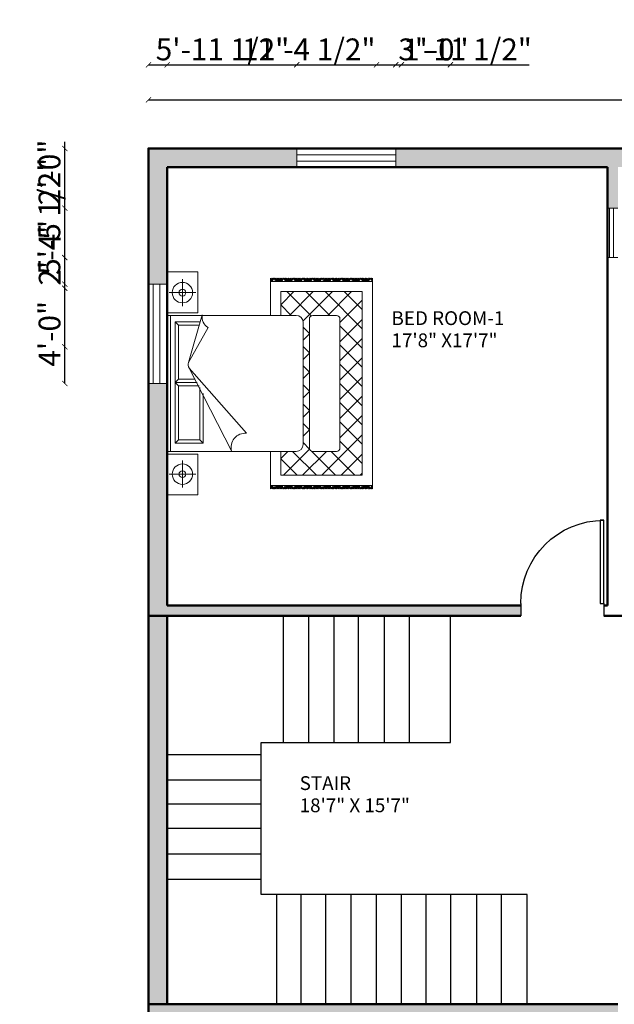
# Model space of a CAD drawing. Units: inches. Extents: x 1549 to 2410, y 1378 to 2139.
# Tile 2 of 6: x 1627 to 1913, y 1657 to 2131. Entities that reach past the tile are written whole.
import ezdxf

# ---------------------------------------------------------------- set-up
doc = ezdxf.new("R2010")
doc.units = ezdxf.units.IN
for name, color, linetype, lineweight in [('A-ANNO-DIMS', 2, 'Continuous', 18), ('A-AREA-IDEN', 7, 'Continuous', 18), ('A-DOOR', 4, 'Continuous', 25), ('A-FLOR-STRS', 3, 'Continuous', 25), ('A-FURN', 8, 'Continuous', 18), ('A-WALL', 7, 'Continuous', 50), ('WINDOW', 2, 'Continuous', 18)]:
    doc.layers.add(name, color=color, linetype=linetype, lineweight=lineweight)
doc.layers.add('A-WALL-PATT', color=18, linetype='Continuous', lineweight=13, true_color=0x000000)
doc.styles.get("Standard").update_dxf_attribs({"font": 'arial.ttf'})
doc.dimstyles.new('ISO-25', dxfattribs={"dimtxt": 10.5, "dimasz": 2.5, "dimexe": 1.25, "dimexo": 0.625, "dimtad": 1, "dimdec": 0, "dimlunit": 4, "dimtxsty": 'Standard', "dimblk": 'ARCHTICK', "dimcen": 2.5, "dimse1": 1, "dimse2": 1, "dimclrd": 1, "dimclrt": 3, "dimadec": 0, "dimazin": 0, "dimtfac": 1, "dimtdec": 0, "dimtmove": 0, "dimatfit": 3, "dimfxl": 1, "dimarcsym": 0})

# ---------------------------------------------------------------- blocks, each defined once
blk = doc.blocks.new('*U3')
for p, q in [((0, 0), (0, -6)), ((40, 0), (40, -6))]:
    blk.add_line(p, q)
blk.add_lwpolyline([(0, 0), (0, 40), (1.75, 40), (1.75, 0)], close=True)
blk.add_arc((0, 0), 40, 0, 90)
blk = doc.blocks.new('A$C4CB008C5')
for p, q in [((0, 3.019), (0.6, 3.019)), ((0, 2.569), (0, 3.019)), ((0.304, 2.6), (0.304, 2.992)), ((0.6, 3.019), (0.6, 2.569)), ((0.64, 1.121), (0.64, 3.021)), ((0.64, 3.021), (2.64, 3.021)), ((0.64, 2.971), (2.64, 2.971)), ((0.759, 2.905), (2.547, 2.905)), ((0.759, 2.489), (0.759, 2.905)), ((0.759, 2.905), (0.809, 2.855)), ((1.603, 2.855), (1.653, 2.905)), ((1.653, 2.905), (1.653, 2.579)), ((1.653, 2.905), (1.703, 2.855)), ((2.497, 2.855), (2.547, 2.905)), ((2.547, 2.905), (2.547, 2.54)), ((2.64, 3.021), (2.64, 1.121)), ((3.279, 3.019), (2.679, 3.019)), ((2.679, 3.019), (2.679, 2.569)), ((2.975, 2.6), (2.975, 2.992)), ((3.279, 2.569), (3.279, 3.019)), ((0.106, 2.796), (0.503, 2.796)), ((0.809, 2.855), (1.603, 2.855)), ((0.809, 2.539), (0.809, 2.855)), ((1.603, 2.855), (1.603, 2.551)), ((1.703, 2.855), (1.703, 2.607)), ((1.703, 2.855), (2.497, 2.855)), ((2.497, 2.855), (2.497, 2.556)), ((3.174, 2.796), (2.776, 2.796)), ((0.64, 2.071), (1.866, 2.698)), ((0.906, 1.854), (1.866, 2.698)), ((1.946, 2.705), (2.646, 2.507)), ((1.946, 2.705), (2.46, 2.418)), ((0.6, 2.569), (0, 2.569)), ((0.809, 2.539), (0.759, 2.489)), ((1.49, 2.489), (0.759, 2.489)), ((1.58, 2.539), (0.809, 2.539)), ((2.679, 2.569), (3.279, 2.569)), ((0.907, 1.867), (0.919, 1.867)), ((0.09, 1.5), (0.64, 1.5)), ((0.09, 1.491), (0.099, 1.5)), ((0.09, 1.473), (0.116, 1.5)), ((0.09, 1.456), (0.134, 1.5)), ((0.09, 1.474), (0.09, 1.475)), ((0.09, 1.438), (0.126, 1.474)), ((0.117, 1.43), (0.09, 1.457)), ((0.14, 1.46), (0.108, 1.492)), ((0.14, 1.478), (0.118, 1.5)), ((0.14, 1.496), (0.135, 1.5)), ((0.14, 0), (0.14, 1.5)), ((2.64, 1.5), (3.19, 1.5)), ((3.14, 1.496), (3.144, 1.5)), ((3.14, 1.478), (3.162, 1.5)), ((3.14, 1.5), (3.14, 0)), ((3.14, 1.46), (3.171, 1.492)), ((3.19, 1.456), (3.145, 1.5)), ((3.19, 1.438), (3.154, 1.474)), ((3.162, 1.43), (3.19, 1.457)), ((3.19, 1.473), (3.163, 1.5)), ((3.19, 1.491), (3.181, 1.5)), ((3.189, 1.474), (3.19, 1.475)), ((0.14, 1.389), (0.09, 1.439)), ((0.09, 1.42), (0.099, 1.43)), ((0.14, 1.372), (0.09, 1.422)), ((0.09, 1.368), (0.14, 1.417)), ((0.14, 1.354), (0.09, 1.404)), ((0.09, 1.35), (0.14, 1.4)), ((0.14, 1.336), (0.09, 1.386)), ((0.09, 1.332), (0.14, 1.382)), ((0.09, 1.314), (0.14, 1.364)), ((0.09, 1.297), (0.126, 1.333)), ((0.09, 1.333), (0.09, 1.333)), ((0.117, 1.288), (0.09, 1.316)), ((0.14, 1.319), (0.108, 1.35)), ((0.117, 1.412), (0.14, 1.435)), ((0.14, 1.442), (0.135, 1.448)), ((0.14, 1.301), (0.135, 1.306)), ((0.29, 1.108), (0.532, 1.35)), ((0.29, 0.15), (0.29, 1.35)), ((0.29, 1.35), (0.64, 1.35)), ((0.674, 0.926), (0.29, 1.31)), ((0.64, 1.243), (0.533, 1.35)), ((2.64, 1.195), (2.795, 1.35)), ((2.64, 1.35), (2.99, 1.35)), ((2.99, 1.156), (2.795, 1.35)), ((2.99, 1.35), (2.99, 0.15)), ((3.14, 1.442), (3.145, 1.448)), ((3.14, 1.389), (3.19, 1.439)), ((3.162, 1.412), (3.14, 1.435)), ((3.14, 1.372), (3.19, 1.422)), ((3.189, 1.368), (3.14, 1.417)), ((3.14, 1.354), (3.19, 1.404)), ((3.19, 1.35), (3.14, 1.4)), ((3.14, 1.336), (3.19, 1.386)), ((3.19, 1.332), (3.14, 1.382)), ((3.19, 1.314), (3.14, 1.364)), ((3.14, 1.319), (3.171, 1.35)), ((3.14, 1.301), (3.145, 1.306)), ((3.19, 1.297), (3.154, 1.333)), ((3.162, 1.288), (3.19, 1.316)), ((3.19, 1.42), (3.18, 1.43)), ((3.189, 1.333), (3.19, 1.333)), ((0.14, 1.248), (0.09, 1.298)), ((0.09, 1.279), (0.099, 1.288)), ((0.14, 1.23), (0.09, 1.28)), ((0.09, 1.227), (0.14, 1.276)), ((0.14, 1.213), (0.09, 1.263)), ((0.09, 1.208), (0.14, 1.258)), ((0.14, 1.195), (0.09, 1.245)), ((0.09, 1.19), (0.14, 1.24)), ((0.09, 1.173), (0.14, 1.223)), ((0.09, 1.191), (0.09, 1.192)), ((0.09, 1.155), (0.126, 1.191)), ((0.117, 1.147), (0.09, 1.174)), ((0.14, 1.177), (0.108, 1.209)), ((0.117, 1.271), (0.14, 1.294)), ((0.14, 1.16), (0.135, 1.165)), ((0.29, 0.825), (0.64, 1.175)), ((2.632, 0.904), (2.99, 1.262)), ((2.99, 0.873), (2.64, 1.223)), ((3.14, 1.248), (3.19, 1.298)), ((3.162, 1.271), (3.14, 1.294)), ((3.14, 1.23), (3.19, 1.28)), ((3.189, 1.227), (3.14, 1.276)), ((3.14, 1.213), (3.19, 1.263)), ((3.19, 1.208), (3.14, 1.258)), ((3.14, 1.195), (3.19, 1.245)), ((3.19, 1.19), (3.14, 1.24)), ((3.19, 1.173), (3.14, 1.223)), ((3.14, 1.177), (3.171, 1.209)), ((3.14, 1.16), (3.145, 1.165)), ((3.19, 1.155), (3.154, 1.191)), ((3.162, 1.147), (3.19, 1.174)), ((3.19, 1.279), (3.18, 1.288)), ((3.189, 1.191), (3.19, 1.192)), ((0.14, 1.107), (0.09, 1.157)), ((0.09, 1.137), (0.099, 1.147)), ((0.14, 1.089), (0.09, 1.139)), ((0.09, 1.085), (0.14, 1.134)), ((0.14, 1.071), (0.09, 1.121)), ((0.09, 1.067), (0.14, 1.117)), ((0.14, 1.054), (0.09, 1.104)), ((0.09, 1.049), (0.14, 1.099)), ((0.09, 1.031), (0.14, 1.081)), ((0.09, 1.05), (0.09, 1.051)), ((0.09, 1.014), (0.126, 1.05)), ((0.117, 1.006), (0.09, 1.033)), ((0.14, 0.965), (0.09, 1.015)), ((0.14, 1.036), (0.108, 1.067)), ((0.117, 1.129), (0.14, 1.152)), ((0.14, 1.018), (0.135, 1.023)), ((0.64, 0.677), (0.29, 1.027)), ((0.673, 0.925), (0.769, 1.021)), ((2.54, 1.021), (0.74, 1.021)), ((0.955, 0.928), (0.861, 1.021)), ((0.959, 0.928), (1.052, 1.021)), ((1.238, 0.928), (1.144, 1.021)), ((1.241, 0.928), (1.335, 1.021)), ((1.52, 0.928), (1.427, 1.021)), ((1.524, 0.928), (1.618, 1.021)), ((1.803, 0.928), (1.71, 1.021)), ((1.807, 0.928), (1.9, 1.021)), ((2.086, 0.928), (1.993, 1.021)), ((2.09, 0.928), (2.183, 1.021)), ((2.369, 0.928), (2.276, 1.021)), ((2.373, 0.928), (2.466, 1.021)), ((2.99, 0.59), (2.557, 1.023)), ((3.14, 1.107), (3.19, 1.157)), ((3.162, 1.129), (3.14, 1.152)), ((3.14, 1.089), (3.19, 1.139)), ((3.189, 1.085), (3.14, 1.134)), ((3.14, 1.071), (3.19, 1.121)), ((3.19, 1.067), (3.14, 1.117)), ((3.14, 1.054), (3.19, 1.104)), ((3.19, 1.049), (3.14, 1.099)), ((3.19, 1.031), (3.14, 1.081)), ((3.14, 1.036), (3.171, 1.067)), ((3.14, 1.018), (3.145, 1.023)), ((3.14, 0.965), (3.19, 1.015)), ((3.19, 1.014), (3.154, 1.05)), ((3.162, 1.006), (3.19, 1.033)), ((3.19, 1.137), (3.18, 1.147)), ((3.189, 1.05), (3.19, 1.051)), ((0.09, 0.996), (0.099, 1.006)), ((0.14, 0.948), (0.09, 0.998)), ((0.09, 0.944), (0.14, 0.993)), ((0.14, 0.93), (0.09, 0.98)), ((0.09, 0.925), (0.14, 0.975)), ((0.14, 0.912), (0.09, 0.962)), ((0.09, 0.908), (0.14, 0.958)), ((0.09, 0.89), (0.14, 0.94)), ((0.09, 0.908), (0.09, 0.909)), ((0.09, 0.872), (0.126, 0.908)), ((0.117, 0.864), (0.09, 0.891)), ((0.14, 0.824), (0.09, 0.874)), ((0.14, 0.894), (0.108, 0.926)), ((0.117, 0.988), (0.14, 1.011)), ((0.117, 0.847), (0.14, 0.869)), ((0.14, 0.877), (0.135, 0.882)), ((0.29, 0.542), (0.643, 0.895)), ((0.64, 0.878), (0.64, 0.528)), ((0.69, 0.928), (2.59, 0.928)), ((2.64, 0.629), (2.99, 0.979)), ((2.64, 0.878), (2.64, 0.528)), ((3.162, 0.988), (3.14, 1.011)), ((3.14, 0.948), (3.19, 0.998)), ((3.189, 0.944), (3.14, 0.993)), ((3.14, 0.93), (3.19, 0.98)), ((3.19, 0.925), (3.14, 0.975)), ((3.14, 0.912), (3.19, 0.962)), ((3.19, 0.908), (3.14, 0.958)), ((3.19, 0.89), (3.14, 0.94)), ((3.14, 0.894), (3.171, 0.926)), ((3.14, 0.877), (3.145, 0.882)), ((3.14, 0.824), (3.19, 0.874)), ((3.162, 0.847), (3.14, 0.869)), ((3.19, 0.872), (3.154, 0.908)), ((3.162, 0.864), (3.19, 0.891)), ((3.19, 0.996), (3.18, 1.006)), ((3.189, 0.908), (3.19, 0.909)), ((0.09, 0.855), (0.099, 0.864)), ((0.14, 0.806), (0.09, 0.856)), ((0.09, 0.802), (0.14, 0.852)), ((0.14, 0.788), (0.09, 0.838)), ((0.09, 0.784), (0.14, 0.834)), ((0.14, 0.771), (0.09, 0.821)), ((0.09, 0.766), (0.14, 0.816)), ((0.09, 0.749), (0.14, 0.799)), ((0.09, 0.767), (0.09, 0.768)), ((0.09, 0.731), (0.126, 0.767)), ((0.117, 0.723), (0.09, 0.75)), ((0.14, 0.682), (0.09, 0.732)), ((0.14, 0.753), (0.108, 0.785)), ((0.117, 0.705), (0.14, 0.728)), ((0.14, 0.735), (0.135, 0.74)), ((0.884, 0.15), (0.29, 0.744)), ((3.14, 0.806), (3.19, 0.856)), ((3.189, 0.802), (3.14, 0.852)), ((3.14, 0.788), (3.19, 0.838)), ((3.19, 0.784), (3.14, 0.834)), ((3.14, 0.771), (3.19, 0.821)), ((3.19, 0.766), (3.14, 0.816)), ((3.19, 0.749), (3.14, 0.799)), ((3.14, 0.753), (3.171, 0.785)), ((3.14, 0.735), (3.145, 0.74)), ((3.14, 0.682), (3.19, 0.732)), ((3.162, 0.705), (3.14, 0.728)), ((3.19, 0.731), (3.154, 0.767)), ((3.162, 0.723), (3.19, 0.75)), ((3.19, 0.855), (3.18, 0.864)), ((3.189, 0.767), (3.19, 0.768)), ((0.09, 0.713), (0.099, 0.723)), ((0.14, 0.665), (0.09, 0.715)), ((0.09, 0.661), (0.14, 0.71)), ((0.14, 0.647), (0.09, 0.697)), ((0.09, 0.642), (0.14, 0.692)), ((0.14, 0.629), (0.09, 0.679)), ((0.09, 0.625), (0.14, 0.675)), ((0.09, 0.607), (0.14, 0.657)), ((0.09, 0.589), (0.126, 0.626)), ((0.09, 0.626), (0.09, 0.626)), ((0.117, 0.581), (0.09, 0.609)), ((0.14, 0.541), (0.09, 0.591)), ((0.09, 0.572), (0.099, 0.581)), ((0.14, 0.612), (0.108, 0.643)), ((0.117, 0.564), (0.14, 0.586)), ((0.14, 0.594), (0.135, 0.599)), ((0.29, 0.259), (0.64, 0.609)), ((2.443, 0.15), (2.99, 0.696)), ((2.99, 0.307), (2.64, 0.657)), ((3.14, 0.665), (3.19, 0.715)), ((3.189, 0.661), (3.14, 0.71)), ((3.14, 0.647), (3.19, 0.697)), ((3.19, 0.642), (3.14, 0.692)), ((3.14, 0.629), (3.19, 0.679)), ((3.19, 0.625), (3.14, 0.675)), ((3.19, 0.607), (3.14, 0.657)), ((3.14, 0.612), (3.171, 0.643)), ((3.14, 0.594), (3.145, 0.599)), ((3.14, 0.541), (3.19, 0.591)), ((3.162, 0.564), (3.14, 0.586)), ((3.19, 0.589), (3.154, 0.626)), ((3.162, 0.581), (3.19, 0.609)), ((3.19, 0.713), (3.18, 0.723)), ((3.19, 0.572), (3.18, 0.581)), ((3.189, 0.626), (3.19, 0.626)), ((0.14, 0.523), (0.09, 0.573)), ((0.09, 0.519), (0.14, 0.569)), ((0.14, 0.506), (0.09, 0.556)), ((0.09, 0.501), (0.14, 0.551)), ((0.14, 0.488), (0.09, 0.538)), ((0.09, 0.483), (0.14, 0.533)), ((0.09, 0.466), (0.14, 0.516)), ((0.09, 0.484), (0.09, 0.485)), ((0.09, 0.448), (0.126, 0.484)), ((0.117, 0.44), (0.09, 0.467)), ((0.14, 0.399), (0.09, 0.449)), ((0.09, 0.43), (0.099, 0.44)), ((0.14, 0.47), (0.108, 0.502)), ((0.117, 0.422), (0.14, 0.445)), ((0.14, 0.453), (0.135, 0.458)), ((0.601, 0.15), (0.29, 0.462)), ((0.463, 0.15), (0.791, 0.478)), ((0.69, 0.478), (2.59, 0.478)), ((0.746, 0.15), (1.074, 0.478)), ((1.167, 0.15), (0.839, 0.478)), ((1.029, 0.15), (1.357, 0.478)), ((1.45, 0.15), (1.122, 0.478)), ((1.312, 0.15), (1.64, 0.478)), ((1.733, 0.15), (1.405, 0.478)), ((1.595, 0.15), (1.923, 0.478)), ((2.016, 0.15), (1.688, 0.478)), ((1.878, 0.15), (2.206, 0.478)), ((2.298, 0.15), (1.97, 0.478)), ((2.16, 0.15), (2.488, 0.478)), ((2.581, 0.15), (2.253, 0.478)), ((2.864, 0.15), (2.536, 0.478)), ((3.14, 0.523), (3.19, 0.573)), ((3.189, 0.519), (3.14, 0.569)), ((3.14, 0.506), (3.19, 0.556)), ((3.19, 0.501), (3.14, 0.551)), ((3.14, 0.488), (3.19, 0.538)), ((3.19, 0.483), (3.14, 0.533)), ((3.19, 0.466), (3.14, 0.516)), ((3.14, 0.47), (3.171, 0.502)), ((3.14, 0.453), (3.145, 0.458)), ((3.14, 0.399), (3.19, 0.449)), ((3.162, 0.422), (3.14, 0.445)), ((3.19, 0.448), (3.154, 0.484)), ((3.162, 0.44), (3.19, 0.467)), ((3.19, 0.43), (3.18, 0.44)), ((3.189, 0.484), (3.19, 0.485)), ((0.14, 0.382), (0.09, 0.432)), ((0.09, 0.378), (0.14, 0.427)), ((0.14, 0.364), (0.09, 0.414)), ((0.09, 0.36), (0.14, 0.41)), ((0.14, 0.346), (0.09, 0.396)), ((0.09, 0.342), (0.14, 0.392)), ((0.09, 0.324), (0.14, 0.374)), ((0.09, 0.307), (0.126, 0.343)), ((0.09, 0.343), (0.09, 0.343)), ((0.117, 0.299), (0.09, 0.326)), ((0.14, 0.258), (0.09, 0.308)), ((0.09, 0.289), (0.099, 0.299)), ((0.14, 0.24), (0.09, 0.29)), ((0.14, 0.329), (0.108, 0.36)), ((0.117, 0.281), (0.14, 0.304)), ((0.14, 0.311), (0.135, 0.316)), ((2.726, 0.15), (2.99, 0.414)), ((3.14, 0.382), (3.19, 0.432)), ((3.189, 0.378), (3.14, 0.427)), ((3.14, 0.364), (3.19, 0.414)), ((3.19, 0.36), (3.14, 0.41)), ((3.14, 0.346), (3.19, 0.396)), ((3.19, 0.342), (3.14, 0.392)), ((3.19, 0.324), (3.14, 0.374)), ((3.14, 0.329), (3.171, 0.36)), ((3.14, 0.311), (3.145, 0.316)), ((3.14, 0.258), (3.19, 0.308)), ((3.162, 0.281), (3.14, 0.304)), ((3.14, 0.24), (3.19, 0.29)), ((3.19, 0.307), (3.154, 0.343)), ((3.162, 0.299), (3.19, 0.326)), ((3.19, 0.289), (3.18, 0.299)), ((3.189, 0.343), (3.19, 0.343)), ((0.09, 0.237), (0.14, 0.286)), ((0.14, 0.223), (0.09, 0.273)), ((0.09, 0.218), (0.14, 0.268)), ((0.14, 0.205), (0.09, 0.255)), ((0.09, 0.201), (0.14, 0.251)), ((0.09, 0.183), (0.14, 0.233)), ((0.09, 0.201), (0.09, 0.202)), ((0.09, 0.165), (0.126, 0.201)), ((0.117, 0.157), (0.09, 0.184)), ((0.14, 0.117), (0.09, 0.167)), ((0.09, 0.148), (0.099, 0.157)), ((0.14, 0.099), (0.09, 0.149)), ((0.14, 0.187), (0.108, 0.219)), ((0.117, 0.139), (0.14, 0.162)), ((0.14, 0.17), (0.135, 0.175)), ((0.318, 0.15), (0.29, 0.179)), ((2.99, 0.15), (0.29, 0.15)), ((3.189, 0.237), (3.14, 0.286)), ((3.14, 0.223), (3.19, 0.273)), ((3.19, 0.218), (3.14, 0.268)), ((3.14, 0.205), (3.19, 0.255)), ((3.19, 0.201), (3.14, 0.251)), ((3.19, 0.183), (3.14, 0.233)), ((3.14, 0.187), (3.171, 0.219)), ((3.14, 0.17), (3.145, 0.175)), ((3.14, 0.117), (3.19, 0.167)), ((3.162, 0.139), (3.14, 0.162)), ((3.14, 0.099), (3.19, 0.149)), ((3.19, 0.165), (3.154, 0.201)), ((3.162, 0.157), (3.19, 0.184)), ((3.19, 0.148), (3.18, 0.157)), ((3.189, 0.201), (3.19, 0.202)), ((0.09, 0.095), (0.14, 0.144)), ((0.14, 0.081), (0.09, 0.131)), ((0.09, 0.077), (0.14, 0.127)), ((0.14, 0.064), (0.09, 0.114)), ((0.09, 0.059), (0.14, 0.109)), ((0.09, 0.041), (0.14, 0.091)), ((0.09, 0.06), (0.09, 0.061)), ((0.09, 0.024), (0.126, 0.06)), ((0.117, 0.016), (0.09, 0.043)), ((0.115, 0), (0.09, 0.025)), ((0.09, 0.006), (0.099, 0.016)), ((0.097, 0), (0.09, 0.008)), ((0.14, 0.046), (0.108, 0.078)), ((0.119, 0), (0.14, 0.021)), ((0.14, 0.028), (0.135, 0.033)), ((0.137, 0), (0.14, 0.003)), ((3.189, 0.095), (3.14, 0.144)), ((3.14, 0.081), (3.19, 0.131)), ((3.19, 0.077), (3.14, 0.127)), ((3.14, 0.064), (3.19, 0.114)), ((3.19, 0.059), (3.14, 0.109)), ((3.19, 0.041), (3.14, 0.091)), ((3.14, 0.046), (3.171, 0.078)), ((3.14, 0.028), (3.145, 0.033)), ((3.16, 0), (3.14, 0.021)), ((3.143, 0), (3.14, 0.003)), ((3.19, 0.024), (3.154, 0.06)), ((3.162, 0.016), (3.19, 0.043)), ((3.164, 0), (3.19, 0.025)), ((3.19, 0.006), (3.18, 0.016)), ((3.182, 0), (3.19, 0.008)), ((3.189, 0.06), (3.19, 0.061)), ((0.09, 0), (3.19, 0))]:
    blk.add_line(p, q)
for centre, radius in [((0.304, 2.796), 0.15), ((2.975, 2.796), 0.15), ((0.304, 2.796), 0.05), ((2.975, 2.796), 0.05)]:
    blk.add_circle(centre, radius)
for centre, radius, start, end in [((1.915, 2.61), 0.1, 71.7215, 119.0799), ((2.626, 2.31), 0.198, 84.1725, 146.9889), ((0.7, 1.873), 0.207, 354.6422, 106.9775), ((0.74, 1.121), 0.1, 180, 270), ((2.54, 1.121), 0.1, 270, 0), ((0.69, 0.878), 0.05, 90, 180), ((2.59, 0.878), 0.05, 0, 90), ((0.69, 0.528), 0.05, 180, 270), ((2.59, 0.528), 0.05, 270, 0)]:
    blk.add_arc(centre, radius, start, end)
blk = doc.blocks.new('_ArchTick')
at = {"color": 0, "linetype": 'ByBlock', "const_width": 0.15}
blk.add_lwpolyline([(-0.5, -0.5), (0.5, 0.5)], dxfattribs=at)
blk = doc.blocks.new('*D13')
at = {"layer": 'A-ANNO-DIMS', "color": 0, "lineweight": -2, "transparency": 16777216}
blk.add_line((1688.62, 2092.38), (2309.62, 2092.38), dxfattribs=at)
at = {"layer": 'Defpoints', "color": 0, "transparency": 16777216}
for p in [(2309.62, 2092.38), (1688.62, 2069.01), (2309.62, 2069.01)]:
    blk.add_point(p, dxfattribs=at)
at = {"layer": 'A-ANNO-DIMS', "color": 0, "lineweight": -2, "transparency": 16777216, "xscale": 2.5, "yscale": 2.5, "zscale": 2.5, "rotation": 180}
blk.add_blockref('_ArchTick', (1688.62, 2092.38), dxfattribs=at)
at = {"layer": 'A-ANNO-DIMS', "color": 0, "lineweight": -2, "transparency": 16777216, "xscale": 2.5, "yscale": 2.5, "zscale": 2.5}
blk.add_blockref('_ArchTick', (2309.62, 2092.38), dxfattribs=at)
at = {"layer": 'A-ANNO-DIMS', "color": 0, "transparency": 16777216, "insert": (1999.12, 2098.36), "char_height": 10.5, "attachment_point": 5}
blk.add_mtext('51\'-9"', dxfattribs=at)
blk = doc.blocks.new('*D33')
at = {"layer": 'A-ANNO-DIMS', "color": 1, "lineweight": -2, "transparency": 16777216}
blk.add_line((1688.62, 2109.26), (1760, 2109.26), dxfattribs=at)
at = {"layer": 'Defpoints', "color": 0, "transparency": 16777216}
for p in [(1760, 2109.26), (1688.62, 2069.01), (1760, 2069.01)]:
    blk.add_point(p, dxfattribs=at)
at = {"layer": 'A-ANNO-DIMS', "color": 1, "lineweight": -2, "transparency": 16777216, "xscale": 2.5, "yscale": 2.5, "zscale": 2.5, "rotation": 180}
blk.add_blockref('_ArchTick', (1688.62, 2109.26), dxfattribs=at)
at = {"layer": 'A-ANNO-DIMS', "color": 1, "lineweight": -2, "transparency": 16777216, "xscale": 2.5, "yscale": 2.5, "zscale": 2.5}
blk.add_blockref('_ArchTick', (1760, 2109.26), dxfattribs=at)
at = {"layer": 'A-ANNO-DIMS', "color": 3, "transparency": 16777216, "insert": (1724.31, 2115.32), "char_height": 10.5, "attachment_point": 5}
blk.add_mtext('5\'-11 1/2"', dxfattribs=at)
blk = doc.blocks.new('*D34')
at = {"layer": 'A-ANNO-DIMS', "color": 1, "lineweight": -2, "transparency": 16777216}
for p, q in [((1760, 2109.26), (1807.68, 2109.26)), ((1807.68, 2109.26), (1871.96, 2109.26))]:
    blk.add_line(p, q, dxfattribs=at)
at = {"layer": 'Defpoints', "color": 0, "transparency": 16777216}
for p in [(1807.68, 2109.26), (1760, 2069.01), (1807.68, 2069.01)]:
    blk.add_point(p, dxfattribs=at)
at = {"layer": 'A-ANNO-DIMS', "color": 1, "lineweight": -2, "transparency": 16777216, "xscale": 2.5, "yscale": 2.5, "zscale": 2.5, "rotation": 180}
blk.add_blockref('_ArchTick', (1760, 2109.26), dxfattribs=at)
at = {"layer": 'A-ANNO-DIMS', "color": 1, "lineweight": -2, "transparency": 16777216, "xscale": 2.5, "yscale": 2.5, "zscale": 2.5}
blk.add_blockref('_ArchTick', (1807.68, 2109.26), dxfattribs=at)
at = {"layer": 'A-ANNO-DIMS', "color": 3, "transparency": 16777216, "insert": (1841.07, 2115.32), "char_height": 10.5, "attachment_point": 5}
blk.add_mtext('3\'-11 1/2"', dxfattribs=at)
blk = doc.blocks.new('*D37')
at = {"layer": 'A-ANNO-DIMS', "color": 1, "lineweight": -2, "transparency": 16777216}
blk.add_line((1648.37, 1955.9), (1648.37, 2003.68), dxfattribs=at)
at = {"layer": 'Defpoints', "color": 0, "transparency": 16777216}
for p in [(1648.37, 2003.68), (1688.62, 2003.68), (1688.62, 1955.9)]:
    blk.add_point(p, dxfattribs=at)
at = {"layer": 'A-ANNO-DIMS', "color": 1, "lineweight": -2, "transparency": 16777216, "xscale": 2.5, "yscale": 2.5, "zscale": 2.5}
for p, rotation in [((1648.37, 2003.68), 90), ((1648.37, 1955.9), 270)]:
    blk.add_blockref('_ArchTick', p, dxfattribs=dict(at, rotation=rotation))
at = {"layer": 'A-ANNO-DIMS', "color": 3, "transparency": 16777216, "insert": (1642.38, 1979.79), "char_height": 10.5, "attachment_point": 5, "rotation": 90}
blk.add_mtext('4\'-0"', dxfattribs=at)
blk = doc.blocks.new('*D38')
at = {"layer": 'A-ANNO-DIMS', "color": 1, "lineweight": -2, "transparency": 16777216}
blk.add_line((1648.37, 2003.68), (1648.37, 2069.01), dxfattribs=at)
at = {"layer": 'Defpoints', "color": 0, "transparency": 16777216}
for p in [(1648.37, 2069.01), (1688.62, 2069.01), (1688.62, 2003.68)]:
    blk.add_point(p, dxfattribs=at)
at = {"layer": 'A-ANNO-DIMS', "color": 1, "lineweight": -2, "transparency": 16777216, "xscale": 2.5, "yscale": 2.5, "zscale": 2.5}
for p, rotation in [((1648.37, 2069.01), 90), ((1648.37, 2003.68), 270)]:
    blk.add_blockref('_ArchTick', p, dxfattribs=dict(at, rotation=rotation))
at = {"layer": 'A-ANNO-DIMS', "color": 3, "transparency": 16777216, "insert": (1642.31, 2036.35), "char_height": 10.5, "attachment_point": 5, "rotation": 90}
blk.add_mtext('5\'-5 1/2"', dxfattribs=at)
blk = doc.blocks.new('*D51')
at = {"layer": 'A-ANNO-DIMS', "color": 1, "lineweight": -2, "transparency": 16777216}
for p, q in [((1648.37, 2001.66), (1648.37, 2033.51)), ((1648.37, 1973.56), (1648.37, 2001.66))]:
    blk.add_line(p, q, dxfattribs=at)
at = {"layer": 'Defpoints', "color": 0, "transparency": 16777216}
for p in [(1648.37, 2001.66), (1914.62, 2001.66), (1914.62, 1973.56)]:
    blk.add_point(p, dxfattribs=at)
at = {"layer": 'A-ANNO-DIMS', "color": 1, "lineweight": -2, "transparency": 16777216, "xscale": 2.5, "yscale": 2.5, "zscale": 2.5}
for p, rotation in [((1648.37, 2001.66), 90), ((1648.37, 1973.56), 270)]:
    blk.add_blockref('_ArchTick', p, dxfattribs=dict(at, rotation=rotation))
at = {"layer": 'A-ANNO-DIMS', "color": 3, "transparency": 16777216, "insert": (1642.47, 2018.83), "char_height": 10.5, "attachment_point": 5, "rotation": 90}
blk.add_mtext('2\'-4"', dxfattribs=at)
blk = doc.blocks.new('*D59')
at = {"layer": 'A-ANNO-DIMS', "color": 1, "lineweight": -2, "transparency": 16777216}
blk.add_line((2400.7, 1782.99), (2400.7, 1844.01), dxfattribs=at)
at = {"layer": 'Defpoints', "color": 0, "transparency": 16777216}
for p in [(1833.98, 1844.01), (2400.7, 1844.01), (1833.98, 1782.99)]:
    blk.add_point(p, dxfattribs=at)
at = {"layer": 'A-ANNO-DIMS', "color": 1, "lineweight": -2, "transparency": 16777216, "xscale": 2.5, "yscale": 2.5, "zscale": 2.5}
for p, rotation in [((2400.7, 1844.01), 90), ((2400.7, 1782.99), 270)]:
    blk.add_blockref('_ArchTick', p, dxfattribs=dict(at, rotation=rotation))
at = {"layer": 'A-ANNO-DIMS', "color": 3, "transparency": 16777216, "insert": (2394.72, 1813.5), "char_height": 10.5, "attachment_point": 5, "rotation": 90}
blk.add_mtext('5\'-1"', dxfattribs=at)
blk = doc.blocks.new('*D60')
at = {"layer": 'A-ANNO-DIMS', "color": 1, "lineweight": -2, "transparency": 16777216}
blk.add_line((2400.7, 1657.01), (2400.7, 1709.88), dxfattribs=at)
at = {"layer": 'Defpoints', "color": 0, "transparency": 16777216}
for p in [(1870.93, 1709.88), (2400.7, 1709.88), (1870.93, 1657.01)]:
    blk.add_point(p, dxfattribs=at)
at = {"layer": 'A-ANNO-DIMS', "color": 1, "lineweight": -2, "transparency": 16777216, "xscale": 2.5, "yscale": 2.5, "zscale": 2.5}
for p, rotation in [((2400.7, 1709.88), 90), ((2400.7, 1657.01), 270)]:
    blk.add_blockref('_ArchTick', p, dxfattribs=dict(at, rotation=rotation))
at = {"layer": 'A-ANNO-DIMS', "color": 3, "transparency": 16777216, "insert": (2394.74, 1683.45), "char_height": 10.5, "attachment_point": 5, "rotation": 90}
blk.add_mtext('4\'-5"', dxfattribs=at)
blk = doc.blocks.new('*D61')
at = {"layer": 'A-ANNO-DIMS', "color": 1, "lineweight": -2, "transparency": 16777216}
for p, q in [((1697.62, 1387.76), (1742.95, 1387.76)), ((1742.95, 1387.76), (1799.07, 1387.76))]:
    blk.add_line(p, q, dxfattribs=at)
at = {"layer": 'Defpoints', "color": 0, "transparency": 16777216}
for p in [(1697.62, 1764.95), (1742.95, 1764.95), (1742.95, 1387.76)]:
    blk.add_point(p, dxfattribs=at)
at = {"layer": 'A-ANNO-DIMS', "color": 1, "lineweight": -2, "transparency": 16777216, "xscale": 2.5, "yscale": 2.5, "zscale": 2.5, "rotation": 180}
blk.add_blockref('_ArchTick', (1697.62, 1387.76), dxfattribs=at)
at = {"layer": 'A-ANNO-DIMS', "color": 1, "lineweight": -2, "transparency": 16777216, "xscale": 2.5, "yscale": 2.5, "zscale": 2.5}
blk.add_blockref('_ArchTick', (1742.95, 1387.76), dxfattribs=at)
at = {"layer": 'A-ANNO-DIMS', "color": 3, "transparency": 16777216, "insert": (1772.26, 1393.82), "char_height": 10.5, "attachment_point": 5}
blk.add_mtext('3\'-9 1/2"', dxfattribs=at)
blk = doc.blocks.new('*D63')
at = {"layer": 'A-ANNO-DIMS', "color": 1, "lineweight": -2, "transparency": 16777216}
blk.add_line((1697.62, 2109.26), (1833.98, 2109.26), dxfattribs=at)
at = {"layer": 'Defpoints', "color": 0, "transparency": 16777216}
for p in [(1833.98, 2109.26), (1697.62, 1844.01), (1833.98, 1844.01)]:
    blk.add_point(p, dxfattribs=at)
at = {"layer": 'A-ANNO-DIMS', "color": 1, "lineweight": -2, "transparency": 16777216, "xscale": 2.5, "yscale": 2.5, "zscale": 2.5, "rotation": 180}
blk.add_blockref('_ArchTick', (1697.62, 2109.26), dxfattribs=at)
at = {"layer": 'A-ANNO-DIMS', "color": 1, "lineweight": -2, "transparency": 16777216, "xscale": 2.5, "yscale": 2.5, "zscale": 2.5}
blk.add_blockref('_ArchTick', (1833.98, 2109.26), dxfattribs=at)
at = {"layer": 'A-ANNO-DIMS', "color": 3, "transparency": 16777216, "insert": (1765.8, 2115.32), "char_height": 10.5, "attachment_point": 5}
blk.add_mtext('11\'-4 1/2"', dxfattribs=at)
blk = doc.blocks.new('*D64')
at = {"layer": 'A-ANNO-DIMS', "color": 1, "lineweight": -2, "transparency": 16777216}
for p, q in [((1798.39, 2109.26), (1810.39, 2109.26)), ((1810.39, 2109.26), (1841.06, 2109.26))]:
    blk.add_line(p, q, dxfattribs=at)
at = {"layer": 'Defpoints', "color": 0, "transparency": 16777216}
for p in [(1810.39, 2109.26), (1798.39, 1709.88), (1810.39, 1709.88)]:
    blk.add_point(p, dxfattribs=at)
at = {"layer": 'A-ANNO-DIMS', "color": 1, "lineweight": -2, "transparency": 16777216, "xscale": 2.5, "yscale": 2.5, "zscale": 2.5, "rotation": 180}
blk.add_blockref('_ArchTick', (1798.39, 2109.26), dxfattribs=at)
at = {"layer": 'A-ANNO-DIMS', "color": 1, "lineweight": -2, "transparency": 16777216, "xscale": 2.5, "yscale": 2.5, "zscale": 2.5}
blk.add_blockref('_ArchTick', (1810.39, 2109.26), dxfattribs=at)
at = {"layer": 'A-ANNO-DIMS', "color": 3, "transparency": 16777216, "insert": (1826.97, 2115.25), "char_height": 10.5, "attachment_point": 5}
blk.add_mtext('1\'-0"', dxfattribs=at)
blk = doc.blocks.new('*D65')
at = {"layer": 'A-ANNO-DIMS', "color": 1, "lineweight": -2, "transparency": 16777216}
for p, q in [((1648.37, 2040.27), (1648.37, 2072.12)), ((1648.37, 2016.45), (1648.37, 2040.27))]:
    blk.add_line(p, q, dxfattribs=at)
at = {"layer": 'Defpoints', "color": 0, "transparency": 16777216}
for p in [(1648.37, 2040.27), (1909.62, 2040.27), (1909.62, 2016.45)]:
    blk.add_point(p, dxfattribs=at)
at = {"layer": 'A-ANNO-DIMS', "color": 1, "lineweight": -2, "transparency": 16777216, "xscale": 2.5, "yscale": 2.5, "zscale": 2.5}
for p, rotation in [((1648.37, 2040.27), 90), ((1648.37, 2016.45), 270)]:
    blk.add_blockref('_ArchTick', p, dxfattribs=dict(at, rotation=rotation))
at = {"layer": 'A-ANNO-DIMS', "color": 3, "transparency": 16777216, "insert": (1642.38, 2057.44), "char_height": 10.5, "attachment_point": 5, "rotation": 90}
blk.add_mtext('2\'-0"', dxfattribs=at)

msp = doc.modelspace()

# ---------------------------------------------------------------- hatches: boundary and pattern name
at = {"layer": 'A-WALL-PATT'}
h = msp.add_hatch(color=256, dxfattribs=at)
h.dxf.hatch_style = 1
h.paths.add_polyline_path([(1760, 2069.01), (1688.62, 2069.01), (1688.62, 2003.68), (1697.62, 2003.68), (1697.62, 2060.01), (1760, 2060.01)])
h.paths.add_polyline_path([(2309.62, 2069.01), (1807.68, 2069.01), (1807.68, 2060.01), (1909.62, 2060.01), (1909.62, 2040.27), (1914.62, 2040.27), (1914.62, 2060.01), (2082.62, 2060.01), (2082.62, 2043.41), (2087.62, 2043.41), (2087.62, 2060.01), (2300.62, 2060.01), (2300.62, 2006.22), (2309.62, 2006.22)])
h.paths.add_polyline_path([(1914.62, 1607.36), (1909.62, 1607.36), (1909.62, 1437.01), (1914.62, 1437.01)])
h.paths.add_polyline_path([(1697.62, 1536.06), (1688.62, 1536.06), (1688.62, 1428.01), (1745.28, 1428.01), (1745.28, 1437.01), (1697.62, 1437.01)])
h.paths.add_polyline_path([(2130.61, 1437.01), (2082.62, 1437.01), (2082.62, 1428.01), (2130.61, 1428.01)])
h.paths.add_polyline_path([(2309.62, 1544.51), (2302.25, 1544.51), (2302.25, 1524.81), (2300.62, 1524.81), (2300.62, 1523.51), (2302.17, 1523.51), (2302.17, 1503.88), (2300.62, 1503.88), (2300.62, 1437.01), (2193.34, 1437.01), (2193.34, 1428.01), (2309.62, 1428.01)])
h.paths.add_polyline_path([(2309.62, 1708.66), (2300.62, 1708.66), (2300.62, 1657.01), (2293.7, 1657.01), (2293.7, 1652.01), (2300.62, 1652.01), (2300.62, 1611.18), (2302.17, 1611.18), (2302.17, 1597.64), (2309.62, 1597.64)])
h.paths.add_polyline_path([(2309.62, 1777.38), (2300.62, 1777.38), (2300.62, 1737.9), (2309.62, 1737.9)])
h.paths.add_polyline_path([(2300.62, 1757.01), (2168.62, 1757.01), (2168.62, 1795.96), (2163.62, 1795.96), (2163.62, 1657.01), (2082.62, 1657.01), (2082.62, 1641.99), (2087.62, 1641.99), (2087.62, 1652.01), (2253.7, 1652.01), (2253.7, 1657.01), (2168.62, 1657.01), (2168.62, 1752.01), (2300.62, 1752.01)])
h.paths.add_polyline_path([(2309.62, 1957.79), (2300.62, 1957.79), (2300.62, 1935.33), (2300.62, 1824.93), (2309.62, 1824.93)])
h.paths.add_polyline_path([(2300.62, 1849.01), (2137.17, 1849.01), (2137.17, 1844.01), (2163.62, 1844.01), (2163.62, 1835.96), (2168.62, 1835.96), (2168.62, 1844.01), (2300.62, 1844.01)])
h.paths.add_polyline_path([(2211.06, 1800.23), (2261.76, 1800.23), (2261.76, 1810.41), (2211.06, 1810.41)], flags=9)
h.paths.add_polyline_path([(2211.1, 1811.05), (2239.18, 1811.05), (2239.18, 1821.02), (2211.1, 1821.02)], flags=9)
h.paths.add_polyline_path([(2187.84, 1718.73), (2233.38, 1718.73), (2233.38, 1728.91), (2187.84, 1728.91)], flags=25)
h.paths.add_polyline_path([(2187.88, 1729.56), (2215.96, 1729.56), (2215.96, 1739.52), (2187.88, 1739.52)], flags=25)
h.paths.add_polyline_path([(1720.01, 1609.74), (1775.87, 1609.74), (1775.87, 1619.93), (1720.01, 1619.93)], flags=9)
h.paths.add_polyline_path([(1719.99, 1620.4), (1782.23, 1620.4), (1782.23, 1630.72), (1719.99, 1630.72)], flags=9)
h.paths.add_polyline_path([(2092.97, 1541.04), (2148.83, 1541.04), (2148.83, 1551.23), (2092.97, 1551.23)], flags=9)
h.paths.add_polyline_path([(2092.94, 1551.69), (2155.19, 1551.69), (2155.19, 1562.02), (2092.94, 1562.02)], flags=9)
h.paths.add_polyline_path([(1759.73, 1747.67), (1815.59, 1747.67), (1815.59, 1757.85), (1759.73, 1757.85)], flags=9)
h.paths.add_polyline_path([(1759.71, 1758.32), (1790.48, 1758.32), (1790.48, 1768.63), (1759.71, 1768.63)], flags=9)
h.paths.add_polyline_path([(1940.79, 1793.43), (1996.65, 1793.43), (1996.65, 1803.61), (1940.79, 1803.61)], flags=9)
h.paths.add_polyline_path([(1940.77, 1804.08), (2006.11, 1804.08), (2006.11, 1814.4), (1940.77, 1814.4)], flags=9)
h.paths.add_polyline_path([(2094.62, 1963.23), (2150.43, 1963.23), (2150.43, 1973.25), (2094.62, 1973.25)], flags=9)
h.paths.add_polyline_path([(2094.57, 1973.75), (2156.81, 1973.75), (2156.81, 1984.07), (2094.57, 1984.07)], flags=9)
h.paths.add_polyline_path([(1943.36, 1930.19), (2000.28, 1930.19), (2000.28, 1940.37), (1943.36, 1940.37)], flags=9)
h.paths.add_polyline_path([(1943.34, 1940.85), (1987.53, 1940.85), (1987.53, 1951.15), (1943.34, 1951.15)], flags=9)
h.paths.add_polyline_path([(1803.94, 1971.5), (1857.22, 1971.5), (1857.22, 1981.68), (1803.94, 1981.68)], flags=9)
h.paths.add_polyline_path([(1803.92, 1982.16), (1866.16, 1982.16), (1866.16, 1992.47), (1803.92, 1992.47)], flags=9)
h = msp.add_hatch(color=256, dxfattribs=at)
h.dxf.hatch_style = 1
h.paths.add_polyline_path([(1697.62, 1844.01), (1688.62, 1844.01), (1688.62, 1657.01), (1697.62, 1657.01)])
h.paths.add_polyline_path([(1697.62, 1955.9), (1688.62, 1955.9), (1688.62, 1844.01), (1697.62, 1844.01), (1867.86, 1844.01), (1867.86, 1849.01), (1697.62, 1849.01)])
h.paths.add_polyline_path([(1697.62, 1652.01), (1909.62, 1652.01), (1909.62, 1647.36), (1914.62, 1647.36), (1914.62, 1657.01), (1697.62, 1657.01), (1688.62, 1657.01), (1688.62, 1584.55), (1697.62, 1584.55)])
h.paths.add_polyline_path([(2087.62, 1601.99), (2082.62, 1601.99), (2082.62, 1437.01), (2087.62, 1437.01)])
h.paths.add_polyline_path([(1981.52, 1547.01), (1914.62, 1547.01), (1914.62, 1540.24), (1981.52, 1540.24)])
h.paths.add_polyline_path([(2082.62, 1547.01), (2061.69, 1547.01), (2061.69, 1540.24), (2082.62, 1540.24)])

# ---------------------------------------------------------------- linework, layer by layer
at = {"layer": 'A-FLOR-STRS'}
for p, q in [((1753.59, 1782.99), (1753.59, 1844.01)), ((1765.83, 1782.99), (1765.83, 1844.01)), ((1778.07, 1782.99), (1778.07, 1844.01)), ((1789.81, 1782.99), (1789.81, 1844.01)), ((1802.3, 1782.99), (1802.3, 1844.01)), ((1814.28, 1782.99), (1814.28, 1844.01)), ((1833.98, 1782.99), (1833.98, 1844.01)), ((1742.95, 1709.88), (1742.95, 1782.99)), ((1742.95, 1782.99), (1833.98, 1782.99)), ((1742.95, 1777.05), (1697.62, 1777.05)), ((1742.95, 1764.95), (1697.62, 1764.95)), ((1742.95, 1753.42), (1697.62, 1753.42)), ((1742.95, 1741.57), (1697.62, 1741.57)), ((1742.95, 1729.26), (1697.62, 1729.26)), ((1742.95, 1717.13), (1697.62, 1717.13)), ((1870.93, 1709.88), (1742.95, 1709.88)), ((1750.48, 1657.01), (1750.48, 1709.88)), ((1762.16, 1657.01), (1762.16, 1709.88)), ((1774.09, 1657.01), (1774.09, 1709.88)), ((1786.27, 1657.01), (1786.27, 1709.88)), ((1786.27, 1657.01), (1786.27, 1709.88)), ((1798.39, 1657.01), (1798.39, 1709.88)), ((1810.39, 1657.01), (1810.39, 1709.88)), ((1822.32, 1657.01), (1822.32, 1709.88)), ((1834.25, 1657.01), (1834.25, 1709.88)), ((1846.68, 1657.01), (1846.68, 1709.88)), ((1858.61, 1657.01), (1858.61, 1709.88)), ((1870.93, 1657.01), (1870.93, 1709.88))]:
    msp.add_line(p, q, dxfattribs=at)
at = {"layer": 'A-WALL'}
for p, q in [((1697.62, 2060.01), (1909.62, 2060.01)), ((1697.62, 1849.01), (1697.62, 2060.01)), ((1909.62, 1849.01), (1909.62, 2060.01)), ((1697.62, 1849.01), (1867.86, 1849.01)), ((1907.86, 1849.01), (1909.62, 1849.01)), ((1697.62, 1844.01), (1688.62, 1844.01)), ((1697.62, 1844.01), (1867.86, 1844.01)), ((1697.62, 1657.01), (1697.62, 1844.01)), ((1697.62, 1844.01), (1697.62, 1844.01)), ((1907.86, 1844.01), (1923.02, 1844.01)), ((1697.62, 1657.01), (1688.62, 1657.01)), ((1697.62, 1657.01), (1914.62, 1657.01))]:
    msp.add_line(p, q, dxfattribs=at)
msp.add_lwpolyline([(1914.62, 1428.01), (1688.62, 1428.01), (1688.62, 2069.01), (2309.62, 2069.01), (2309.62, 1428.01), (2082.62, 1428.01)], dxfattribs=at)
at = {"layer": 'WINDOW'}
for p, q in [((1760, 2069.01), (1760, 2060.01)), ((1807.68, 2069.01), (1760, 2069.01)), ((1807.68, 2060.01), (1807.68, 2069.01)), ((1807.68, 2065.86), (1760, 2065.86)), ((1807.68, 2062.91), (1760, 2062.91)), ((1760, 2060.01), (1807.68, 2060.01)), ((1914.62, 2040.27), (1909.62, 2040.27)), ((1909.62, 2040.27), (1909.62, 2016.45)), ((1910.52, 2016.45), (1910.52, 2040.27)), ((1912.57, 2016.45), (1912.57, 2040.27)), ((1909.62, 2016.45), (1914.62, 2016.45)), ((1697.62, 2003.68), (1688.62, 2003.68)), ((1688.62, 2003.68), (1688.62, 1955.9)), ((1690.97, 1955.9), (1690.97, 2003.68)), ((1694.14, 1955.9), (1694.14, 2003.68)), ((1697.62, 1955.9), (1697.62, 2003.68)), ((1688.62, 1955.9), (1697.62, 1955.9))]:
    msp.add_line(p, q, dxfattribs=at)

# ---------------------------------------------------------------- block references
at = {"layer": 'A-DOOR', "xscale": -1}
msp.add_blockref('*U3', (1907.86, 1850.01), dxfattribs=at)
at = {"layer": 'A-FURN', "xscale": 32.72052747801291, "yscale": 32.72052747801291, "zscale": 32.72052747801291, "rotation": 90}
msp.add_blockref('A$C4CB008C5', (1796.48, 1902.25), dxfattribs=at)

# ---------------------------------------------------------------- texts
at = {"layer": 'A-AREA-IDEN'}
for s, height, p in [('BED ROOM-1', 6.645, (1805.64, 1983.99)), ('17\'8" X17\'7"', 6.6455, (1805.64, 1973.31)), ('STAIR', 6.645, (1761.43, 1760.16)), ('18\'7" X 15\'7"', 6.6455, (1761.43, 1749.48))]:
    msp.add_text(s, height=height, dxfattribs=at).set_placement(p)

# ---------------------------------------------------------------- dimensions: what is measured, and where the dimension line sits
at = {"layer": 'A-ANNO-DIMS'}
for base, p1, p2, override, picture, middle in [((1760, 2109.26), (1688.62, 2069.01), (1760, 2069.01), {"dimdec": 1, "dimlfac": 1, "dimrnd": 0, "dimzin": 1, "dimdsep": 46, "dimlunit": 4, "dimfrac": 2}, '*D33', (1724.31, 2115.32)), ((1833.98, 2109.26), (1697.62, 1844.01), (1833.98, 1844.01), {"dimdec": 1, "dimlfac": 1, "dimrnd": 0, "dimzin": 1, "dimdsep": 46, "dimlunit": 4, "dimfrac": 2}, '*D63', (1765.8, 2115.32)), ((1807.68, 2109.26), (1760, 2069.01), (1807.68, 2069.01), {"dimdec": 1, "dimlfac": 1, "dimrnd": 0, "dimzin": 1, "dimdsep": 46, "dimlunit": 4, "dimfrac": 2}, '*D34', (1841.07, 2115.32)), ((1810.39, 2109.26), (1798.39, 1709.88), (1810.39, 1709.88), {"dimdec": 1, "dimlfac": 1, "dimrnd": 0, "dimzin": 1, "dimdsep": 46, "dimlunit": 4, "dimfrac": 2}, '*D64', (1826.97, 2115.25)), ((2309.62, 2092.38), (1688.62, 2069.01), (2309.62, 2069.01), {"dimclrd": 0, "dimclre": 0, "dimclrt": 0}, '*D13', (1999.12, 2098.36)), ((1742.95, 1387.76), (1697.62, 1764.95), (1742.95, 1764.95), {"dimdec": 1, "dimlfac": 1, "dimrnd": 0, "dimzin": 1, "dimdsep": 46, "dimlunit": 4, "dimfrac": 2}, '*D61', (1772.26, 1393.82))]:
    dim = msp.add_linear_dim(base=base, p1=p1, p2=p2, dimstyle='ISO-25', override=override, dxfattribs=at)
    dim.commit()
    dim.dimension.update_dxf_attribs({"geometry": picture, "text_midpoint": middle})
for base, p1, p2, picture, middle in [((1648.37, 2040.27), (1909.62, 2016.45), (1909.62, 2040.27), '*D65', (1642.38, 2057.44)), ((1648.37, 2069.01), (1688.62, 2003.68), (1688.62, 2069.01), '*D38', (1642.31, 2036.35)), ((1648.37, 2001.66), (1914.62, 1973.56), (1914.62, 2001.66), '*D51', (1642.47, 2018.83)), ((1648.37, 2003.68), (1688.62, 1955.9), (1688.62, 2003.68), '*D37', (1642.38, 1979.79)), ((2400.7, 1844.01), (1833.98, 1782.99), (1833.98, 1844.01), '*D59', (2394.72, 1813.5)), ((2400.7, 1709.88), (1870.93, 1657.01), (1870.93, 1709.88), '*D60', (2394.74, 1683.45))]:
    dim = msp.add_linear_dim(base=base, p1=p1, p2=p2, angle=90, dimstyle='ISO-25', override={"dimdec": 1, "dimlfac": 1, "dimrnd": 0, "dimzin": 1, "dimdsep": 46, "dimlunit": 4, "dimfrac": 2}, dxfattribs=at)
    dim.commit()
    dim.dimension.update_dxf_attribs({"geometry": picture, "text_midpoint": middle})

doc.saveas('drawing.dxf')
